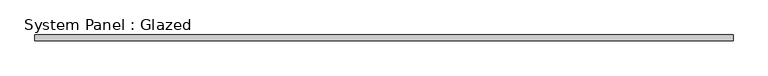
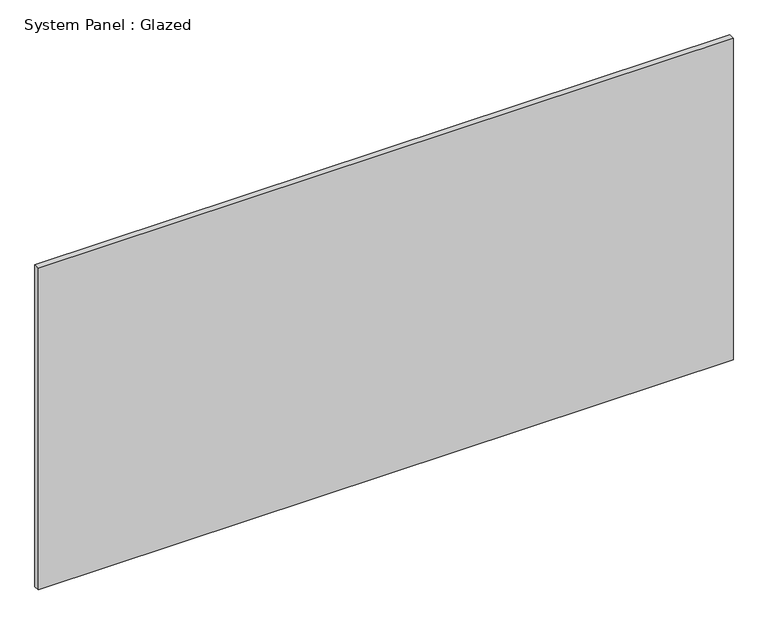
"""IFC4 building model written with IfcOpenShell, lengths in millimetres: plate geometry, System Panel : Glazed."""

from ifc_helpers import new_model, si_unit, origin, origin_with_axes, place, context, project, spatial, polyline, outline, extrude, source, transform, mapped, element, save


def system_panel_glazed_2a6c68b7(model_context):
    return source(origin(), model_context, "Body", "SweptSolid", [
        extrude(outline(polyline([(1492.25, 19.05), (-1492.25, 19.05), (-1492.25, 44.45), (1492.25, 44.45), (1492.25, 19.05)])), origin_with_axes(), (0.0, 0.0, 1.0), 1460.5),
    ])


if __name__ == "__main__":
    model = new_model("IFC4")
    model_context = context("Model", 3, world=origin())
    ifc_project = project(units=[si_unit("LENGTHUNIT", "METRE", prefix="MILLI")], contexts=[model_context])
    site = spatial("IfcSite", under=ifc_project)
    building = spatial("IfcBuilding", under=site)
    placement = place(None, origin())
    system_panel_glazed_shape = system_panel_glazed_2a6c68b7(model_context)
    element("IfcPlate", 1, ObjectType="System Panel : Glazed", at=placement, inside=building, context=model_context, shape_type="MappedRepresentation", body=[
        mapped(system_panel_glazed_shape, transform((0.0, 0.0, 0.0), x_axis=(1.0, 0.0, 0.0), y_axis=(0.0, 1.0, 0.0), z_axis=(0.0, 0.0, 1.0))),
    ])
    save(model, "model.ifc")

# Revit data of these elements
# Type "System Panel : Glazed"
#   Construction Type Id = "GSP4R"
#   Analytic Construction = "1/8 in Pilkington single glazing"
#   Visual Light Transmittance = 0.9
#   Solar Heat Gain Coefficient = 0.86
#   Heat Transfer Coefficient (U) = 1.18115 BTU/(h·ft²·°F)
#   Define Thermal Properties by = 1
# Element 1 (IfcPlate, "System Panel : Glazed")
#   Materials on its faces: "Glass"
# Materials
#   "Glass": class "Glass", colour RGB 0 128 192, transparency 0.75, Description = "Soda Lime Glass", Cost = 0
